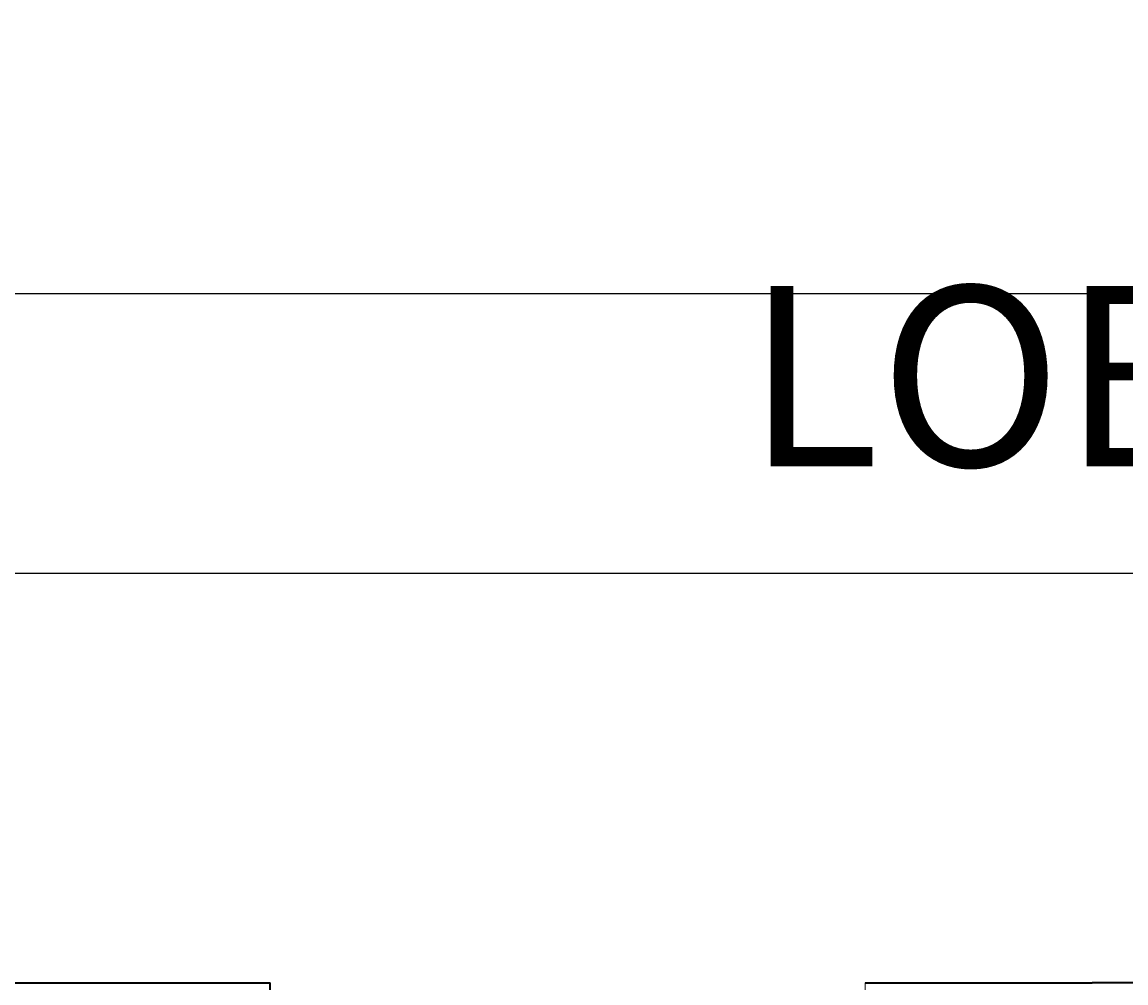
# Model space of a CAD drawing. Units: feet. Extents: x 5816 to 6644, y 25475 to 26788.
# Tile 7 of 23: x 6159 to 6232, y 26094 to 26158. Entities that reach past the tile are written whole.
import ezdxf

# ---------------------------------------------------------------- set-up
doc = ezdxf.new("R2010")
doc.units = ezdxf.units.FT
for name, color, linetype, lineweight in [('A-ANNO-DIMS', 2, 'Continuous', 13), ('A-AREA-IDEN', 7, 'Continuous', 18), ('A-DOOR', 3, 'Continuous', 18), ('A-WALL', 7, 'Continuous', 35)]:
    doc.layers.add(name, color=color, linetype=linetype, lineweight=lineweight)
doc.styles.get("Standard").update_dxf_attribs({"font": 'arial.ttf'})
doc.dimstyles.get("Standard").update_dxf_attribs({"dimtxt": 0.18, "dimasz": 0.18, "dimexe": 0.18, "dimexo": 0.0625, "dimgap": 0.09, "dimtad": 0, "dimtih": 1, "dimtoh": 1, "dimdec": 4, "dimzin": 0, "dimdsep": 46, "dimtxsty": 'Standard', "dimcen": 0.09, "dimadec": 0, "dimazin": 0, "dimtfac": 1, "dimtdec": 4, "dimtofl": 0, "dimtmove": 0, "dimatfit": 3, "dimfxl": 1, "dimtolj": 1, "dimtzin": 0, "dimarcsym": 0})

# ---------------------------------------------------------------- blocks, each defined once
blk = doc.blocks.new('DOOR-FLAT-ENTRY')
blk.add_line((0, 55.131), (0, 0))
blk.add_arc((7.052, 9.007), 46.66, 98.693, 180)
blk = doc.blocks.new('*D60')
at = {"layer": 'A-ANNO-DIMS', "color": 0, "lineweight": -2, "transparency": 16777216}
for p, q in [((6106.978, 26094.399), (6106.978, 26787.915)), ((6107.158, 26787.735), (6224.932, 26787.735)), ((6343.496, 26787.735), (6225.722, 26787.735)), ((6343.676, 26094.399), (6343.676, 26787.915))]:
    blk.add_line(p, q, dxfattribs=at)
at = {"layer": 'A-ANNO-DIMS', "color": 0, "transparency": 16777216}
for points in [[(6107.158, 26787.765), (6107.158, 26787.705), (6106.978, 26787.735)], [(6343.496, 26787.765), (6343.496, 26787.705), (6343.676, 26787.735)]]:
    blk.add_solid(points, dxfattribs=at)
at = {"layer": 'Defpoints', "color": 0, "transparency": 16777216}
for p in [(6343.676, 26787.735), (6106.978, 26094.337), (6343.676, 26094.337)]:
    blk.add_point(p, dxfattribs=at)
at = {"layer": 'A-ANNO-DIMS', "color": 0, "transparency": 16777216, "insert": (6225.327, 26787.735), "char_height": 0.18, "attachment_point": 5}
blk.add_mtext('\\A1;236.7', dxfattribs=at)
blk = doc.blocks.new('*D71')
at = {"layer": 'A-ANNO-DIMS', "color": 0, "lineweight": -2, "transparency": 16777216}
for p, q in [((6343.614, 26140.224), (5815.982, 26140.224)), ((5816.162, 26140.044), (5816.162, 26131.1)), ((5816.162, 26121.792), (5816.162, 26130.736)), ((6343.614, 26121.612), (5815.982, 26121.612))]:
    blk.add_line(p, q, dxfattribs=at)
at = {"layer": 'A-ANNO-DIMS', "color": 0, "transparency": 16777216}
for points in [[(5816.132, 26140.044), (5816.192, 26140.044), (5816.162, 26140.224)], [(5816.132, 26121.792), (5816.192, 26121.792), (5816.162, 26121.612)]]:
    blk.add_solid(points, dxfattribs=at)
at = {"layer": 'Defpoints', "color": 0, "transparency": 16777216}
for p in [(6343.676, 26140.224), (5816.162, 26121.612), (6343.676, 26121.612)]:
    blk.add_point(p, dxfattribs=at)
at = {"layer": 'A-ANNO-DIMS', "color": 0, "transparency": 16777216, "insert": (5816.162, 26130.918), "char_height": 0.18, "attachment_point": 5}
blk.add_mtext('\\A1;18.61', dxfattribs=at)

msp = doc.modelspace()

# ---------------------------------------------------------------- linework, layer by layer
at = {"layer": 'A-WALL'}
for p, q in [((5962.9781, 26094.3368), (6175.0829, 26094.3368)), ((6175.0829, 26085.3298), (6175.0829, 26094.3368)), ((6214.6905, 26094.3368), (6229.8119, 26094.3368)), ((6244.9332, 26094.3368), (6229.8119, 26094.3368))]:
    msp.add_line(p, q, dxfattribs=at)

# ---------------------------------------------------------------- block references
at = {"layer": 'A-DOOR', "extrusion": (0, 0, -1), "zscale": -1, "rotation": 180}
msp.add_blockref('DOOR-FLAT-ENTRY', (-6214.6905, 26094.3368), dxfattribs=at)

# ---------------------------------------------------------------- texts
at = {"layer": 'A-AREA-IDEN'}
msp.add_text('LOBBY', height=12, dxfattribs=at).set_placement((6206.7608, 26128.7481))

# ---------------------------------------------------------------- dimensions: what is measured, and where the dimension line sits
at = {"layer": 'A-ANNO-DIMS'}
dim = msp.add_linear_dim(base=(6343.6763, 26787.7346), p1=(6106.9781, 26094.3368), p2=(6343.6763, 26094.3368), dimstyle='Standard', override={"dimdec": 1, "dimlfac": 1, "dimrnd": 0, "dimzin": 0, "dimdsep": 46, "dimlunit": 2}, dxfattribs=at)
dim.commit()
dim.dimension.update_dxf_attribs({"geometry": '*D60', "text_midpoint": (6225.3272, 26787.7346)})
dim = msp.add_linear_dim(base=(5816.1619, 26121.6124), p1=(6343.6763, 26140.2241), p2=(6343.6763, 26121.6124), angle=90, dimstyle='Standard', override={"dimdec": 2, "dimlfac": 1, "dimrnd": 0, "dimzin": 0, "dimdsep": 46, "dimlunit": 2}, dxfattribs=at)
dim.commit()
dim.dimension.update_dxf_attribs({"geometry": '*D71', "text_midpoint": (5816.1619, 26130.9183)})

doc.saveas('drawing.dxf')
